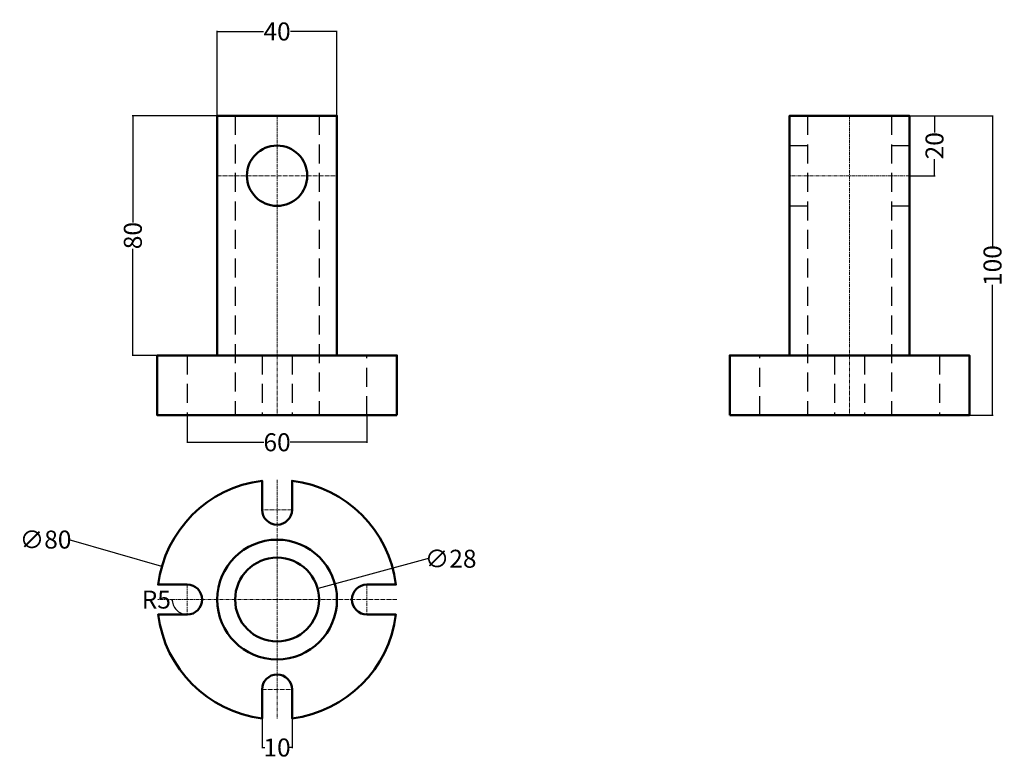
# Model space of a CAD drawing. Units: millimetres. Extents: x 18 to 347, y 6 to 253.
import ezdxf

# ---------------------------------------------------------------- set-up
doc = ezdxf.new("R2010")
doc.units = ezdxf.units.MM
doc.header["$MEASUREMENT"] = 0
doc.linetypes.add('CENTER', pattern=[2, 1.25, -0.25, 0.25, -0.25])
doc.linetypes.add('HIDDEN', pattern=[9.525, 6.35, -3.175])
for name, color, linetype, lineweight in [('M-CNTR', 1, 'CENTER', 18), ('M-DIMS', 2, 'Continuous', 25), ('M-HIDN', 3, 'HIDDEN', 25), ('M-OUTL', 7, 'Continuous', 50)]:
    doc.layers.add(name, color=color, linetype=linetype, lineweight=lineweight)
doc.styles.get("Standard").update_dxf_attribs({"font": 'arial.ttf'})
doc.dimstyles.get("Standard").update_dxf_attribs({"dimtxt": 6, "dimasz": 0.18, "dimexe": 0.18, "dimexo": 0.0625, "dimgap": 0.09, "dimtad": 0, "dimtoh": 1, "dimdec": 0, "dimzin": 0, "dimdsep": 46, "dimtxsty": 'Standard', "dimcen": 0.09, "dimadec": 0, "dimazin": 0, "dimtfac": 1, "dimtdec": 0, "dimtofl": 0, "dimtmove": 0, "dimatfit": 3, "dimfxl": 1, "dimtolj": 1, "dimtzin": 0, "dimarcsym": 0})

# ---------------------------------------------------------------- blocks, each defined once
blk = doc.blocks.new('*D1')
at = {"layer": 'Defpoints', "color": 0, "transparency": 16777216}
for p in [(65.59, 69.96), (142.45, 47.77)]:
    blk.add_point(p, dxfattribs=at)
at = {"layer": 'M-DIMS', "color": 0, "lineweight": -2, "transparency": 16777216}
for p, q in [((34.39, 78.91), (34.57, 78.91)), ((34.57, 78.91), (65.41, 70.01)), ((103.93, 58.87), (104.11, 58.87)), ((104.02, 58.78), (104.02, 58.96))]:
    blk.add_line(p, q, dxfattribs=at)
at = {"layer": 'M-DIMS', "color": 0, "transparency": 16777216}
blk.add_solid([(65.42, 70.04), (65.41, 69.98), (65.59, 69.96)], dxfattribs=at)
at = {"layer": 'M-DIMS', "color": 0, "transparency": 16777216, "insert": (26.75, 78.91), "char_height": 6, "attachment_point": 5}
blk.add_mtext('\\A1;∅80', dxfattribs=at)
blk = doc.blocks.new('*D2')
at = {"layer": 'Defpoints', "color": 0, "transparency": 16777216}
for p in [(117.53, 62.55), (90.51, 55.19)]:
    blk.add_point(p, dxfattribs=at)
at = {"layer": 'M-DIMS', "color": 0, "lineweight": -2, "transparency": 16777216}
for p, q in [((154.12, 72.51), (117.7, 62.59)), ((154.3, 72.51), (154.12, 72.51)), ((103.93, 58.87), (104.11, 58.87)), ((104.02, 58.78), (104.02, 58.96))]:
    blk.add_line(p, q, dxfattribs=at)
at = {"layer": 'M-DIMS', "color": 0, "transparency": 16777216}
blk.add_solid([(117.69, 62.62), (117.71, 62.56), (117.53, 62.55)], dxfattribs=at)
at = {"layer": 'M-DIMS', "color": 0, "transparency": 16777216, "insert": (161.96, 72.51), "char_height": 6, "attachment_point": 5}
blk.add_mtext('\\A1;∅28', dxfattribs=at)
blk = doc.blocks.new('*D3')
at = {"layer": 'Defpoints', "color": 0, "transparency": 16777216}
for p in [(99.02, 19.18), (109.02, 19.18), (109.02, 9.47)]:
    blk.add_point(p, dxfattribs=at)
at = {"layer": 'M-DIMS', "color": 0, "lineweight": -2, "transparency": 16777216}
for p, q in [((99.02, 19.12), (99.02, 9.29)), ((109.02, 19.12), (109.02, 9.29)), ((99.2, 9.47), (99.92, 9.47)), ((108.84, 9.47), (108.11, 9.47))]:
    blk.add_line(p, q, dxfattribs=at)
at = {"layer": 'M-DIMS', "color": 0, "transparency": 16777216}
for points in [[(99.2, 9.5), (99.2, 9.44), (99.02, 9.47)], [(108.84, 9.5), (108.84, 9.44), (109.02, 9.47)]]:
    blk.add_solid(points, dxfattribs=at)
at = {"layer": 'M-DIMS', "color": 0, "transparency": 16777216, "insert": (104.02, 9.47), "char_height": 6, "attachment_point": 5}
blk.add_mtext('\\A1;10', dxfattribs=at)
blk = doc.blocks.new('*D4')
at = {"layer": 'Defpoints', "color": 0, "transparency": 16777216}
for p in [(69.02, 58.87), (74.02, 58.87)]:
    blk.add_point(p, dxfattribs=at)
at = {"layer": 'M-DIMS', "color": 0, "lineweight": -2, "transparency": 16777216}
for p, q in [((68.66, 58.87), (68.84, 58.87)), ((73.93, 58.87), (74.11, 58.87)), ((74.02, 58.78), (74.02, 58.96))]:
    blk.add_line(p, q, dxfattribs=at)
blk.add_arc((74.02, 58.87), 5, 177.9374, 269.2838, dxfattribs=at)
at = {"layer": 'M-DIMS', "color": 0, "transparency": 16777216}
blk.add_solid([(68.84, 58.9), (68.84, 58.84), (69.02, 58.87)], dxfattribs=at)
at = {"layer": 'M-DIMS', "color": 0, "transparency": 16777216, "insert": (63.71, 58.87), "char_height": 6, "attachment_point": 5}
blk.add_mtext('\\A1;R5', dxfattribs=at)
blk = doc.blocks.new('*D5')
at = {"layer": 'Defpoints', "color": 0, "transparency": 16777216}
for p in [(74.02, 120.41), (134.02, 120.41), (134.02, 111.4)]:
    blk.add_point(p, dxfattribs=at)
at = {"layer": 'M-DIMS', "color": 0, "lineweight": -2, "transparency": 16777216}
for p, q in [((74.02, 120.35), (74.02, 111.22)), ((134.02, 120.35), (134.02, 111.22)), ((74.2, 111.4), (99.62, 111.4)), ((133.84, 111.4), (108.41, 111.4))]:
    blk.add_line(p, q, dxfattribs=at)
at = {"layer": 'M-DIMS', "color": 0, "transparency": 16777216}
for points in [[(74.2, 111.43), (74.2, 111.37), (74.02, 111.4)], [(133.84, 111.43), (133.84, 111.37), (134.02, 111.4)]]:
    blk.add_solid(points, dxfattribs=at)
at = {"layer": 'M-DIMS', "color": 0, "transparency": 16777216, "insert": (104.02, 111.4), "char_height": 6, "attachment_point": 5}
blk.add_mtext('\\A1;60', dxfattribs=at)
blk = doc.blocks.new('*D6')
at = {"layer": 'Defpoints', "color": 0, "transparency": 16777216}
for p in [(84.02, 220.41), (55.88, 140.41), (84.02, 140.41)]:
    blk.add_point(p, dxfattribs=at)
at = {"layer": 'M-DIMS', "color": 0, "lineweight": -2, "transparency": 16777216}
for p, q in [((83.96, 220.41), (55.7, 220.41)), ((55.88, 220.23), (55.88, 184.8)), ((55.88, 140.59), (55.88, 176.03)), ((83.96, 140.41), (55.7, 140.41))]:
    blk.add_line(p, q, dxfattribs=at)
at = {"layer": 'M-DIMS', "color": 0, "transparency": 16777216}
for points in [[(55.85, 220.23), (55.91, 220.23), (55.88, 220.41)], [(55.85, 140.59), (55.91, 140.59), (55.88, 140.41)]]:
    blk.add_solid(points, dxfattribs=at)
at = {"layer": 'M-DIMS', "color": 0, "transparency": 16777216, "insert": (55.88, 180.41), "char_height": 6, "attachment_point": 5, "rotation": 90}
blk.add_mtext('\\A1;80', dxfattribs=at)
blk = doc.blocks.new('*D7')
at = {"layer": 'Defpoints', "color": 0, "transparency": 16777216}
for p in [(124.02, 248.58), (84.02, 220.41), (124.02, 220.41)]:
    blk.add_point(p, dxfattribs=at)
at = {"layer": 'M-DIMS', "color": 0, "lineweight": -2, "transparency": 16777216}
for p, q in [((84.02, 220.48), (84.02, 248.76)), ((84.2, 248.58), (99.52, 248.58)), ((123.84, 248.58), (108.52, 248.58)), ((124.02, 220.48), (124.02, 248.76))]:
    blk.add_line(p, q, dxfattribs=at)
at = {"layer": 'M-DIMS', "color": 0, "transparency": 16777216}
for points in [[(84.2, 248.61), (84.2, 248.55), (84.02, 248.58)], [(123.84, 248.61), (123.84, 248.55), (124.02, 248.58)]]:
    blk.add_solid(points, dxfattribs=at)
at = {"layer": 'M-DIMS', "color": 0, "transparency": 16777216, "insert": (104.02, 248.58), "char_height": 6, "attachment_point": 5}
blk.add_mtext('\\A1;40', dxfattribs=at)
blk = doc.blocks.new('*D8')
at = {"layer": 'Defpoints', "color": 0, "transparency": 16777216}
for p in [(315.11, 220.41), (315.11, 200.41), (323.46, 200.41)]:
    blk.add_point(p, dxfattribs=at)
at = {"layer": 'M-DIMS', "color": 0, "lineweight": -2, "transparency": 16777216}
for p, q in [((315.17, 220.41), (323.64, 220.41)), ((323.46, 220.23), (323.46, 214.84)), ((323.46, 200.59), (323.46, 205.99)), ((315.17, 200.41), (323.64, 200.41))]:
    blk.add_line(p, q, dxfattribs=at)
at = {"layer": 'M-DIMS', "color": 0, "transparency": 16777216}
for points in [[(323.43, 220.23), (323.49, 220.23), (323.46, 220.41)], [(323.43, 200.59), (323.49, 200.59), (323.46, 200.41)]]:
    blk.add_solid(points, dxfattribs=at)
at = {"layer": 'M-DIMS', "color": 0, "transparency": 16777216, "insert": (323.46, 210.41), "char_height": 6, "attachment_point": 5, "rotation": 90}
blk.add_mtext('\\A1;20', dxfattribs=at)
blk = doc.blocks.new('*D9')
at = {"layer": 'Defpoints', "color": 0, "transparency": 16777216}
for p in [(315.11, 220.41), (335.11, 120.41), (342.82, 120.41)]:
    blk.add_point(p, dxfattribs=at)
at = {"layer": 'M-DIMS', "color": 0, "lineweight": -2, "transparency": 16777216}
for p, q in [((315.17, 220.41), (343, 220.41)), ((342.82, 220.23), (342.82, 176.84)), ((342.82, 120.59), (342.82, 163.99)), ((335.17, 120.41), (343, 120.41))]:
    blk.add_line(p, q, dxfattribs=at)
at = {"layer": 'M-DIMS', "color": 0, "transparency": 16777216}
for points in [[(342.79, 220.23), (342.85, 220.23), (342.82, 220.41)], [(342.79, 120.59), (342.85, 120.59), (342.82, 120.41)]]:
    blk.add_solid(points, dxfattribs=at)
at = {"layer": 'M-DIMS', "color": 0, "transparency": 16777216, "insert": (342.82, 170.41), "char_height": 6, "attachment_point": 5, "rotation": 90}
blk.add_mtext('\\A1;100', dxfattribs=at)

msp = doc.modelspace()

# ---------------------------------------------------------------- linework, layer by layer
at = {"layer": 'M-CNTR'}
for p, q in [((104.02, 220.41), (104.02, 120.29)), ((295.11, 220.41), (295.11, 120.29)), ((84.02, 200.41), (124.02, 200.41)), ((315.11, 200.41), (275.11, 200.41)), ((109.02, 88.87), (99.02, 88.87)), ((74.02, 63.87), (74.02, 53.87)), ((134.02, 63.87), (134.02, 53.87)), ((144.02, 58.87), (64.02, 58.87)), ((99.02, 28.87), (109.02, 28.87))]:
    msp.add_line(p, q, dxfattribs=at)
msp.add_lwpolyline([(104.02, 98.87), (104.02, 58.87), (104.02, 18.87)], dxfattribs=at)
at = {"layer": 'M-HIDN'}
for p, q in [((90.02, 220.41), (90.02, 120.29)), ((118.02, 220.41), (118.02, 120.29)), ((281.11, 220.41), (281.11, 120.29)), ((309.11, 220.41), (309.11, 120.29)), ((275.11, 210.49), (281.11, 210.49)), ((309.11, 210.49), (315.11, 210.49)), ((275.11, 190.34), (281.11, 190.34)), ((309.11, 190.34), (315.11, 190.34)), ((74.02, 140.41), (74.02, 120.41)), ((99.02, 140.41), (99.02, 120.29)), ((109.02, 140.41), (109.02, 120.29)), ((134.02, 120.41), (134.02, 140.41)), ((265.11, 120.41), (265.11, 140.41)), ((290.11, 140.41), (290.11, 120.29)), ((300.11, 140.41), (300.11, 120.29)), ((325.11, 140.41), (325.11, 120.41))]:
    msp.add_line(p, q, dxfattribs=at)
at = {"layer": 'M-OUTL'}
for points in [[(84.02, 140.41), (84.02, 220.41), (124.02, 220.41), (124.02, 140.41)], [(315.11, 140.41), (315.11, 220.41), (275.11, 220.41), (275.11, 140.41)]]:
    msp.add_lwpolyline(points, dxfattribs=at)
for points in [[(144.02, 120.41), (144.02, 140.41), (64.02, 140.41), (64.02, 120.41)], [(255.11, 120.41), (255.11, 140.41), (335.11, 140.41), (335.11, 120.41)]]:
    msp.add_lwpolyline(points, close=True, dxfattribs=at)
msp.add_lwpolyline([(134.02, 63.87), (143.7, 63.87, 0.342564), (109.02, 98.55), (109.02, 88.87, -1), (99.02, 88.87), (99.02, 98.55, 0.342564), (64.33, 63.87), (74.02, 63.87, -1), (74.02, 53.87), (64.33, 53.87, 0.342564), (99.02, 19.18), (99.02, 28.87, -1), (109.02, 28.87), (109.02, 19.18, 0.342564), (143.7, 53.87), (134.02, 53.87, -1)], format="xyb", close=True, dxfattribs=at)
for centre, radius in [((104.02, 200.41), 10.08), ((104.02, 58.87), 20), ((104.02, 58.87), 14)]:
    msp.add_circle(centre, radius, dxfattribs=at)

# ---------------------------------------------------------------- dimensions: what is measured, and where the dimension line sits
at = {"layer": 'M-DIMS'}
for base, p1, p2, picture, middle in [((124.02, 248.58), (84.02, 220.41), (124.02, 220.41), '*D7', (104.02, 248.58)), ((134.02, 111.4), (74.02, 120.41), (134.02, 120.41), '*D5', (104.02, 111.4)), ((109.02, 9.47), (99.02, 19.18), (109.02, 19.18), '*D3', (104.02, 9.47))]:
    dim = msp.add_linear_dim(base=base, p1=p1, p2=p2, dimstyle='Standard', override={"dimclrd": 0, "dimclre": 0, "dimclrt": 0}, dxfattribs=at)
    dim.commit()
    dim.dimension.update_dxf_attribs({"geometry": picture, "text_midpoint": middle})
for base, p1, p2, picture, middle in [((55.88, 140.41), (84.02, 220.41), (84.02, 140.41), '*D6', (55.88, 180.41)), ((323.46, 200.41), (315.11, 220.41), (315.11, 200.41), '*D8', (323.46, 210.41)), ((342.82, 120.41), (315.11, 220.41), (335.11, 120.41), '*D9', (342.82, 170.41))]:
    dim = msp.add_linear_dim(base=base, p1=p1, p2=p2, angle=90, dimstyle='Standard', override={"dimclrd": 0, "dimclre": 0, "dimclrt": 0}, dxfattribs=at)
    dim.commit()
    dim.dimension.update_dxf_attribs({"geometry": picture, "text_midpoint": middle})
for p1, p2, picture, middle in [((142.45, 47.77), (65.59, 69.96), '*D1', (26.75, 78.91)), ((90.51, 55.19), (117.53, 62.55), '*D2', (161.96, 72.51))]:
    dim = msp.add_diameter_dim_2p(p1=p1, p2=p2, dimstyle='Standard', override={"dimclrd": 0, "dimclre": 0, "dimclrt": 0}, dxfattribs=at)
    dim.commit()
    dim.dimension.update_dxf_attribs({"geometry": picture, "text_midpoint": middle, "dimtype": 163})
dim = msp.add_radius_dim(center=(74.02, 58.87), mpoint=(69.02, 58.87), dimstyle='Standard', override={"dimclrd": 0, "dimclre": 0, "dimclrt": 0}, dxfattribs=at)
dim.commit()
dim.dimension.update_dxf_attribs({"geometry": '*D4', "text_midpoint": (63.71, 58.87)})

doc.saveas('drawing.dxf')
